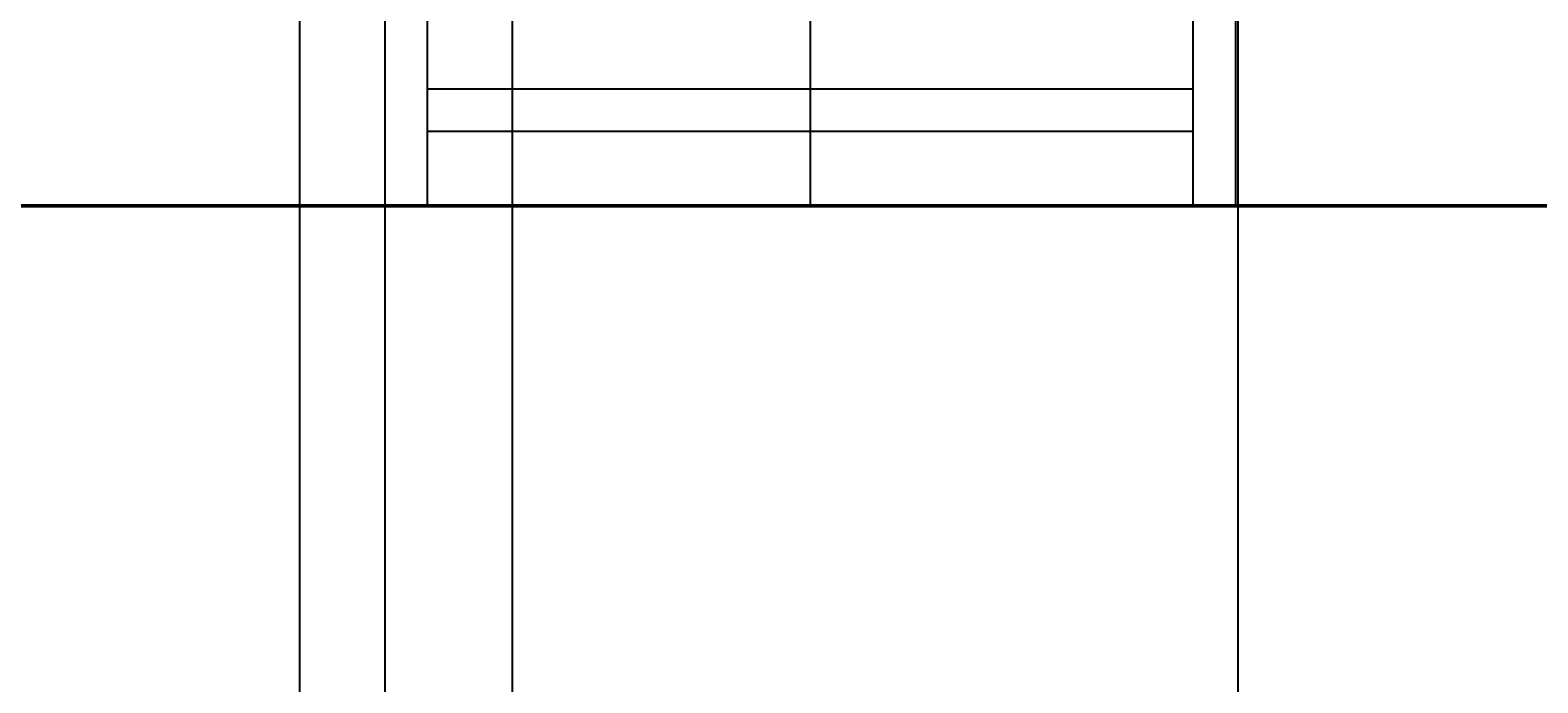
# Model space of a CAD drawing. Units: inches. Extents: x 37 to 824, y -700 to 234.
# Tile 57 of 77: x 193 to 264, y 160 to 190. Entities that reach past the tile are written whole.
import ezdxf

# ---------------------------------------------------------------- set-up
doc = ezdxf.new("R2010")
doc.units = ezdxf.units.IN
doc.header["$MEASUREMENT"] = 0
for name, color, linetype, lineweight in [('A-ANNO-DIMS', 2, 'Continuous', 18), ('A-GLAZ', 4, 'Continuous', 25), ('A-WALL', 2, 'Continuous', 50)]:
    doc.layers.add(name, color=color, linetype=linetype, lineweight=lineweight)
doc.styles.get("Standard").update_dxf_attribs({"font": 'arial.ttf'})
doc.dimstyles.get("Standard").update_dxf_attribs({"dimtxt": 0.18, "dimasz": 0.18, "dimexe": 0.18, "dimexo": 0.0625, "dimgap": 0.09, "dimtad": 0, "dimtih": 1, "dimtoh": 1, "dimdec": 1, "dimzin": 0, "dimdsep": 46, "dimlunit": 4, "dimtxsty": 'Standard', "dimcen": 0.09, "dimadec": 0, "dimazin": 0, "dimtfac": 1, "dimtdec": 1, "dimtofl": 0, "dimtmove": 0, "dimatfit": 3, "dimfxl": 1, "dimtolj": 1, "dimtzin": 0, "dimarcsym": 0})

# ---------------------------------------------------------------- blocks, each defined once
blk = doc.blocks.new('WIN-900')
for p, q in [((0, 9), (0, 0)), ((2, 9), (2, 0)), ((20, 9), (20, 0)), ((38, 9), (38, 0)), ((40, 9), (40, 0)), ((38, 5.5), (2, 5.5)), ((38, 3.5), (2, 3.5))]:
    blk.add_line(p, q)
blk = doc.blocks.new('*D72')
at = {"layer": 'A-ANNO-DIMS', "color": 0, "lineweight": -2, "ltscale": 0.5, "transparency": 16777216}
for p, q in [((170.077, 84.153), (170.077, 234.17)), ((170.257, 233.99), (209.804, 233.99)), ((250.01, 233.99), (210.463, 233.99)), ((250.19, 84.153), (250.19, 234.17))]:
    blk.add_line(p, q, dxfattribs=at)
at = {"layer": 'A-ANNO-DIMS', "color": 0, "ltscale": 0.5, "transparency": 16777216}
for points in [[(170.257, 234.02), (170.257, 233.96), (170.077, 233.99)], [(250.01, 234.02), (250.01, 233.96), (250.19, 233.99)]]:
    blk.add_solid(points, dxfattribs=at)
at = {"layer": 'Defpoints', "color": 0, "ltscale": 0.5, "transparency": 16777216}
for p in [(250.19, 233.99), (170.077, 84.09), (250.19, 84.09)]:
    blk.add_point(p, dxfattribs=at)
at = {"layer": 'A-ANNO-DIMS', "color": 0, "ltscale": 0.5, "transparency": 16777216, "insert": (210.133, 233.99), "char_height": 0.18, "attachment_point": 5}
blk.add_mtext('\\A1;6\'-8"', dxfattribs=at)
blk = doc.blocks.new('*D73')
at = {"layer": 'A-ANNO-DIMS', "color": 0, "lineweight": -2, "ltscale": 0.5, "transparency": 16777216}
for p, q in [((250.19, 84.153), (250.19, 234.17)), ((250.37, 233.99), (269.804, 233.99)), ((289.897, 233.99), (270.463, 233.99)), ((290.077, 81.153), (290.077, 234.17))]:
    blk.add_line(p, q, dxfattribs=at)
at = {"layer": 'A-ANNO-DIMS', "color": 0, "ltscale": 0.5, "transparency": 16777216}
for points in [[(250.37, 234.02), (250.37, 233.96), (250.19, 233.99)], [(289.897, 234.02), (289.897, 233.96), (290.077, 233.99)]]:
    blk.add_solid(points, dxfattribs=at)
at = {"layer": 'Defpoints', "color": 0, "ltscale": 0.5, "transparency": 16777216}
for p in [(290.077, 233.99), (250.19, 84.09), (290.077, 81.09)]:
    blk.add_point(p, dxfattribs=at)
at = {"layer": 'A-ANNO-DIMS', "color": 0, "ltscale": 0.5, "transparency": 16777216, "insert": (270.133, 233.99), "char_height": 0.18, "attachment_point": 5}
blk.add_mtext('\\A1;3\'-4"', dxfattribs=at)
blk = doc.blocks.new('*D84')
at = {"layer": 'A-ANNO-DIMS', "color": 0, "lineweight": -2, "ltscale": 0.5, "transparency": 16777216}
for p, q in [((170.077, -265.847), (170.077, 234.17)), ((170.257, 233.99), (189.748, 233.99)), ((209.897, 233.99), (190.406, 233.99)), ((210.077, -265.847), (210.077, 234.17))]:
    blk.add_line(p, q, dxfattribs=at)
at = {"layer": 'A-ANNO-DIMS', "color": 0, "ltscale": 0.5, "transparency": 16777216}
for points in [[(170.257, 234.02), (170.257, 233.96), (170.077, 233.99)], [(209.897, 234.02), (209.897, 233.96), (210.077, 233.99)]]:
    blk.add_solid(points, dxfattribs=at)
at = {"layer": 'Defpoints', "color": 0, "ltscale": 0.5, "transparency": 16777216}
for p in [(210.077, 233.99), (170.077, -265.91), (210.077, -265.91)]:
    blk.add_point(p, dxfattribs=at)
at = {"layer": 'A-ANNO-DIMS', "color": 0, "ltscale": 0.5, "transparency": 16777216, "insert": (190.077, 233.99), "char_height": 0.18, "attachment_point": 5}
blk.add_mtext('\\A1;3\'-4"', dxfattribs=at)
blk = doc.blocks.new('*D85')
at = {"layer": 'A-ANNO-DIMS', "color": 0, "lineweight": -2, "ltscale": 0.5, "transparency": 16777216}
for p, q in [((170.077, -356.847), (170.077, 234.17)), ((170.257, 233.99), (187.748, 233.99)), ((205.897, 233.99), (188.406, 233.99)), ((206.077, -356.847), (206.077, 234.17))]:
    blk.add_line(p, q, dxfattribs=at)
at = {"layer": 'A-ANNO-DIMS', "color": 0, "ltscale": 0.5, "transparency": 16777216}
for points in [[(170.257, 234.02), (170.257, 233.96), (170.077, 233.99)], [(205.897, 234.02), (205.897, 233.96), (206.077, 233.99)]]:
    blk.add_solid(points, dxfattribs=at)
at = {"layer": 'Defpoints', "color": 0, "ltscale": 0.5, "transparency": 16777216}
for p in [(206.077, 233.99), (170.077, -356.91), (206.077, -356.91)]:
    blk.add_point(p, dxfattribs=at)
at = {"layer": 'A-ANNO-DIMS', "color": 0, "ltscale": 0.5, "transparency": 16777216, "insert": (188.077, 233.99), "char_height": 0.18, "attachment_point": 5}
blk.add_mtext('\\A1;3\'-0"', dxfattribs=at)
blk = doc.blocks.new('*D86')
at = {"layer": 'A-ANNO-DIMS', "color": 0, "lineweight": -2, "ltscale": 0.5, "transparency": 16777216}
for p, q in [((206.077, -356.847), (206.077, 234.17)), ((206.257, 233.99), (210.678, 233.99)), ((215.897, 233.99), (211.476, 233.99)), ((216.077, -356.847), (216.077, 234.17))]:
    blk.add_line(p, q, dxfattribs=at)
at = {"layer": 'A-ANNO-DIMS', "color": 0, "ltscale": 0.5, "transparency": 16777216}
for points in [[(206.257, 234.02), (206.257, 233.96), (206.077, 233.99)], [(215.897, 234.02), (215.897, 233.96), (216.077, 233.99)]]:
    blk.add_solid(points, dxfattribs=at)
at = {"layer": 'Defpoints', "color": 0, "ltscale": 0.5, "transparency": 16777216}
for p in [(216.077, 233.99), (206.077, -356.91), (216.077, -356.91)]:
    blk.add_point(p, dxfattribs=at)
at = {"layer": 'A-ANNO-DIMS', "color": 0, "ltscale": 0.5, "transparency": 16777216, "insert": (211.077, 233.99), "char_height": 0.18, "attachment_point": 5}
blk.add_mtext('\\A1;0\'-10"', dxfattribs=at)
blk = doc.blocks.new('*D87')
at = {"layer": 'A-ANNO-DIMS', "color": 0, "lineweight": -2, "ltscale": 0.5, "transparency": 16777216}
for p, q in [((216.077, -356.847), (216.077, 234.17)), ((216.257, 233.99), (255.747, 233.99)), ((295.897, 233.99), (256.407, 233.99)), ((296.077, -356.847), (296.077, 234.17))]:
    blk.add_line(p, q, dxfattribs=at)
at = {"layer": 'A-ANNO-DIMS', "color": 0, "ltscale": 0.5, "transparency": 16777216}
for points in [[(216.257, 234.02), (216.257, 233.96), (216.077, 233.99)], [(295.897, 234.02), (295.897, 233.96), (296.077, 233.99)]]:
    blk.add_solid(points, dxfattribs=at)
at = {"layer": 'Defpoints', "color": 0, "ltscale": 0.5, "transparency": 16777216}
for p in [(296.077, 233.99), (216.077, -356.91), (296.077, -356.91)]:
    blk.add_point(p, dxfattribs=at)
at = {"layer": 'A-ANNO-DIMS', "color": 0, "ltscale": 0.5, "transparency": 16777216, "insert": (256.077, 233.99), "char_height": 0.18, "attachment_point": 5}
blk.add_mtext('\\A1;6\'-8"', dxfattribs=at)

msp = doc.modelspace()

# ---------------------------------------------------------------- linework, layer by layer
at = {"layer": 'A-WALL'}
msp.add_line((170.077, 182.09), (290.077, 182.09), dxfattribs=at)

# ---------------------------------------------------------------- block references
at = {"layer": 'A-GLAZ', "rotation": 180}
msp.add_blockref('WIN-900', (250.077, 191.091), dxfattribs=at)

# ---------------------------------------------------------------- dimensions: what is measured, and where the dimension line sits
at = {"layer": 'A-ANNO-DIMS', "ltscale": 0.5}
for base, p1, p2, picture, middle in [((250.19, 233.99), (170.077, 84.09), (250.19, 84.09), '*D72', (210.133, 233.99)), ((210.077, 233.99), (170.077, -265.91), (210.077, -265.91), '*D84', (190.077, 233.99)), ((206.077, 233.99), (170.077, -356.91), (206.077, -356.91), '*D85', (188.077, 233.99)), ((216.077, 233.99), (206.077, -356.91), (216.077, -356.91), '*D86', (211.077, 233.99)), ((296.077, 233.99), (216.077, -356.91), (296.077, -356.91), '*D87', (256.077, 233.99)), ((290.077, 233.99), (250.19, 84.09), (290.077, 81.09), '*D73', (270.133, 233.99))]:
    dim = msp.add_linear_dim(base=base, p1=p1, p2=p2, dimstyle='Standard', override={"dimdec": 1, "dimlfac": 1, "dimrnd": 0, "dimzin": 1, "dimdsep": 46, "dimlunit": 4, "dimfrac": 2}, dxfattribs=at)
    dim.commit()
    dim.dimension.update_dxf_attribs({"geometry": picture, "text_midpoint": middle})

doc.saveas('drawing.dxf')
